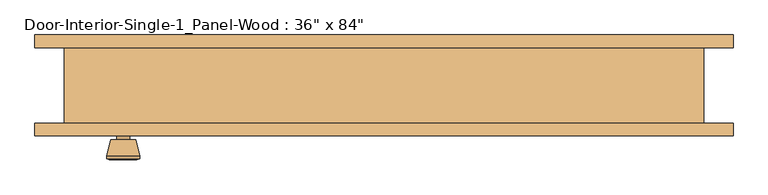
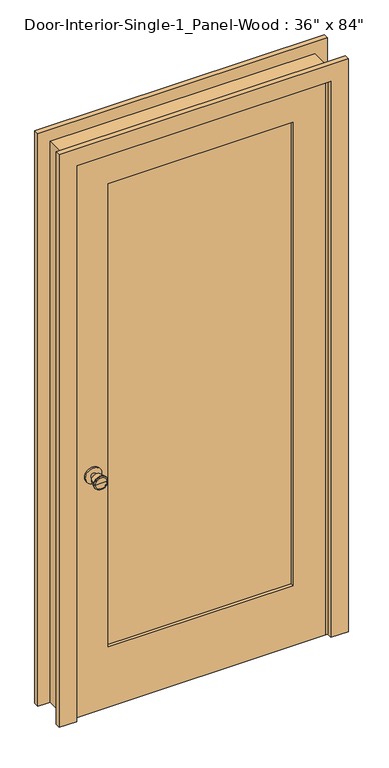
"""IFC4 building model written with IfcOpenShell, lengths in millimetres: door geometry."""

from ifc_helpers import new_model, si_unit, point, frame, frame_2d, origin, place, context, project, spatial, polyline, circle_curve, trimmed, segment, composite_curve, outline, extrude, faceted_brep, source, transform, mapped, element, save
from ifc_brep_helpers import plane_surface, cylinder_surface, revolved_surface, advanced_brep


def door_a3feeac7(model_context):
    return source(origin(), model_context, "Body", "SolidModel", [
        advanced_brep(
        [(-393.7, -13.05, 914.4), (-403.7, -13.05, 914.4), (-383.7, -13.05, 914.4), (-373.2241324, 35.95, 914.4), (-414.1758676, 35.95, 914.4), (-393.7, 35.95, 914.4), (-368.7, 34.1221319, 914.4), (-418.7, 34.1221319, 914.4), (-368.7, 30.6584537, 914.4), (-418.7, 30.6584537, 914.4), (-375.063764, 5.95, 914.4), (-412.336236, 5.95, 914.4), (-383.7, 5.95, 914.4), (-403.7, 5.95, 914.4)],
        [
            (0, 1),
            (1, 2, circle_curve(frame((-393.7, -13.05, 914.4), z_axis=(0.0, -1.0, 0.0), x_axis=(-1.0, 0.0, 0.0)), 10.0)),
            (2, 0),
            (2, 1, circle_curve(frame((-393.7, -13.05, 914.4), z_axis=(0.0, -1.0, 0.0), x_axis=(-1.0, 0.0, 0.0)), 10.0)),
            (3, 4, circle_curve(frame((-393.7, 35.95, 914.4), z_axis=(0.0, 1.0, 0.0), x_axis=(-1.0, 0.0, 0.0)), 20.4758676)),
            (4, 5),
            (5, 3),
            (4, 3, circle_curve(frame((-393.7, 35.95, 914.4), z_axis=(0.0, 1.0, 0.0), x_axis=(-1.0, 0.0, 0.0)), 20.4758676)),
            (6, 7, circle_curve(frame((-393.7, 34.1221319, 914.4), z_axis=(0.0, 1.0, 0.0), x_axis=(-1.0, 0.0, 0.0)), 25.0)),
            (7, 4),
            (3, 6),
            (7, 6, circle_curve(frame((-393.7, 34.1221319, 914.4), z_axis=(0.0, 1.0, 0.0), x_axis=(-1.0, 0.0, 0.0)), 25.0)),
            (8, 9, circle_curve(frame((-393.7, 30.6584537, 914.4), z_axis=(0.0, 1.0, 0.0), x_axis=(-1.0, 0.0, 0.0)), 25.0)),
            (9, 7),
            (6, 8),
            (9, 8, circle_curve(frame((-393.7, 30.6584537, 914.4), z_axis=(0.0, 1.0, 0.0), x_axis=(-1.0, 0.0, 0.0)), 25.0)),
            (10, 11, circle_curve(frame((-393.7, 5.95, 914.4), z_axis=(0.0, 1.0, 0.0), x_axis=(-1.0, 0.0, 0.0)), 18.636236)),
            (11, 9),
            (8, 10),
            (11, 10, circle_curve(frame((-393.7, 5.95, 914.4), z_axis=(0.0, 1.0, 0.0), x_axis=(-1.0, 0.0, 0.0)), 18.636236)),
            (12, 13, circle_curve(frame((-393.7, 5.95, 914.4), z_axis=(0.0, 1.0, 0.0), x_axis=(-1.0, 0.0, 0.0)), 10.0)),
            (13, 11),
            (10, 12),
            (13, 12, circle_curve(frame((-393.7, 5.95, 914.4), z_axis=(0.0, 1.0, 0.0), x_axis=(-1.0, 0.0, 0.0)), 10.0)),
            (1, 13),
            (12, 2),
        ],
        [
            plane_surface(frame((-393.7, -13.05, 914.4), z_axis=(0.0, -1.0, 0.0), x_axis=(-1.0, 0.0, 0.0))),
            plane_surface(frame((-393.7, 35.95, 914.4), z_axis=(0.0, 1.0, 0.0), x_axis=(-1.0, 0.0, 0.0))),
            revolved_surface(polyline([(-414.1758676, 35.95, 914.4), (-418.7, 34.1221319, 914.4)]), (-393.7, -13.05, 914.4), (0.0, -1.0, 0.0)),
            cylinder_surface(frame((-393.7, -13.05, 914.4), z_axis=(0.0, -1.0, 0.0), x_axis=(-1.0, 0.0, 0.0)), 25.0),
            revolved_surface(polyline([(-418.7, 30.6584537, 914.4), (-412.336236, 5.95, 914.4)]), (-393.7, -13.05, 914.4), (0.0, -1.0, 0.0)),
            plane_surface(frame((-393.7, 5.95, 914.4), z_axis=(0.0, -1.0, 0.0), x_axis=(-1.0, 0.0, 0.0))),
            cylinder_surface(frame((-393.7, -13.05, 914.4), z_axis=(0.0, -1.0, 0.0), x_axis=(-1.0, 0.0, 0.0)), 10.0),
        ],
        [
            (0, [[1, 2, 3]]),
            (0, [[-3, 4, -1]]),
            (1, [[5, 6, 7]]),
            (1, [[8, -7, -6]]),
            (2, [[9, 10, -5, 11]]),
            (2, [[12, -11, -8, -10]]),
            (3, [[13, 14, -9, 15]]),
            (3, [[16, -15, -12, -14]]),
            (4, [[17, 18, -13, 19]]),
            (4, [[20, -19, -16, -18]]),
            (5, [[21, 22, -17, 23]]),
            (5, [[24, -23, -20, -22]]),
            (6, [[-2, 25, -21, 26]]),
            (6, [[-4, -26, -24, -25]]),
        ],
    ),
        extrude(outline(composite_curve([segment(trimmed(circle_curve(frame_2d((914.4, -393.7)), 30.0), [point((914.4, -423.7))], [point((914.4, -363.7))], False, "CARTESIAN"), True, "CONTINUOUS"), segment(trimmed(circle_curve(frame_2d((914.4, -393.7)), 30.0), [point((914.4, -363.7))], [point((914.4, -423.7))], False, "CARTESIAN"), True, "CONTINUOUS")], self_intersect=False)), frame((0.0, -19.05, 0.0), z_axis=(0.0, 1.0, 0.0), x_axis=(0.0, 0.0, 1.0)), (0.0, 0.0, 1.0), 6.0),
        advanced_brep(
        [(-393.7, -59.975, 914.4), (-383.7, -59.975, 914.4), (-403.7, -59.975, 914.4), (-373.2241324, -108.975, 914.4), (-393.7, -108.975, 914.4), (-414.1758676, -108.975, 914.4), (-368.7, -107.1471319, 914.4), (-418.7, -107.1471319, 914.4), (-368.7, -103.6834537, 914.4), (-418.7, -103.6834537, 914.4), (-375.063764, -78.975, 914.4), (-412.336236, -78.975, 914.4), (-383.7, -78.975, 914.4), (-403.7, -78.975, 914.4)],
        [
            (0, 1),
            (1, 2, circle_curve(frame((-393.7, -59.975, 914.4), z_axis=(0.0, 1.0, 0.0), x_axis=(-1.0, 0.0, 0.0)), 10.0)),
            (2, 0),
            (2, 1, circle_curve(frame((-393.7, -59.975, 914.4), z_axis=(0.0, 1.0, 0.0), x_axis=(-1.0, 0.0, 0.0)), 10.0)),
            (3, 4),
            (4, 5),
            (5, 3, circle_curve(frame((-393.7, -108.975, 914.4), z_axis=(0.0, -1.0, 0.0), x_axis=(-1.0, 0.0, 0.0)), 20.4758676)),
            (3, 5, circle_curve(frame((-393.7, -108.975, 914.4), z_axis=(0.0, -1.0, 0.0), x_axis=(-1.0, 0.0, 0.0)), 20.4758676)),
            (6, 3),
            (5, 7),
            (7, 6, circle_curve(frame((-393.7, -107.1471319, 914.4), z_axis=(0.0, -1.0, 0.0), x_axis=(-1.0, 0.0, 0.0)), 25.0)),
            (6, 7, circle_curve(frame((-393.7, -107.1471319, 914.4), z_axis=(0.0, -1.0, 0.0), x_axis=(-1.0, 0.0, 0.0)), 25.0)),
            (8, 6),
            (7, 9),
            (9, 8, circle_curve(frame((-393.7, -103.6834537, 914.4), z_axis=(0.0, -1.0, 0.0), x_axis=(-1.0, 0.0, 0.0)), 25.0)),
            (8, 9, circle_curve(frame((-393.7, -103.6834537, 914.4), z_axis=(0.0, -1.0, 0.0), x_axis=(-1.0, 0.0, 0.0)), 25.0)),
            (10, 8),
            (9, 11),
            (11, 10, circle_curve(frame((-393.7, -78.975, 914.4), z_axis=(0.0, -1.0, 0.0), x_axis=(-1.0, 0.0, 0.0)), 18.636236)),
            (10, 11, circle_curve(frame((-393.7, -78.975, 914.4), z_axis=(0.0, -1.0, 0.0), x_axis=(-1.0, 0.0, 0.0)), 18.636236)),
            (12, 10),
            (11, 13),
            (13, 12, circle_curve(frame((-393.7, -78.975, 914.4), z_axis=(0.0, -1.0, 0.0), x_axis=(-1.0, 0.0, 0.0)), 10.0)),
            (12, 13, circle_curve(frame((-393.7, -78.975, 914.4), z_axis=(0.0, -1.0, 0.0), x_axis=(-1.0, 0.0, 0.0)), 10.0)),
            (1, 12),
            (13, 2),
        ],
        [
            plane_surface(frame((-393.7, -59.975, 914.4), z_axis=(0.0, 1.0, 0.0), x_axis=(-1.0, 0.0, 0.0))),
            plane_surface(frame((-393.7, -108.975, 914.4), z_axis=(0.0, -1.0, 0.0), x_axis=(-1.0, 0.0, 0.0))),
            revolved_surface(polyline([(-414.1758676, -108.975, 914.4), (-418.7, -107.1471319, 914.4)]), (-393.7, -59.975, 914.4), (0.0, 1.0, 0.0)),
            cylinder_surface(frame((-393.7, -59.975, 914.4), z_axis=(0.0, 1.0, 0.0), x_axis=(-1.0, 0.0, 0.0)), 25.0),
            revolved_surface(polyline([(-418.7, -103.6834537, 914.4), (-412.336236, -78.975, 914.4)]), (-393.7, -59.975, 914.4), (0.0, 1.0, 0.0)),
            plane_surface(frame((-393.7, -78.975, 914.4), z_axis=(0.0, 1.0, 0.0), x_axis=(-1.0, 0.0, 0.0))),
            cylinder_surface(frame((-393.7, -59.975, 914.4), z_axis=(0.0, 1.0, 0.0), x_axis=(-1.0, 0.0, 0.0)), 10.0),
        ],
        [
            (0, [[1, 2, 3]]),
            (0, [[-3, 4, -1]]),
            (1, [[5, 6, 7]]),
            (1, [[-6, -5, 8]]),
            (2, [[9, -7, 10, 11]]),
            (2, [[-10, -8, -9, 12]]),
            (3, [[13, -11, 14, 15]]),
            (3, [[-14, -12, -13, 16]]),
            (4, [[17, -15, 18, 19]]),
            (4, [[-18, -16, -17, 20]]),
            (5, [[21, -19, 22, 23]]),
            (5, [[-22, -20, -21, 24]]),
            (6, [[25, -23, 26, -2]]),
            (6, [[-26, -24, -25, -4]]),
        ],
    ),
        extrude(outline(composite_curve([segment(trimmed(circle_curve(frame_2d((914.4, -393.7)), 30.0), [point((914.4, -423.7))], [point((914.4, -363.7))], False, "CARTESIAN"), True, "CONTINUOUS"), segment(trimmed(circle_curve(frame_2d((914.4, -393.7)), 30.0), [point((914.4, -363.7))], [point((914.4, -423.7))], False, "CARTESIAN"), True, "CONTINUOUS")], self_intersect=False)), frame((0.0, -59.975, 0.0), z_axis=(0.0, 1.0, 0.0), x_axis=(0.0, 0.0, 1.0)), (0.0, 0.0, 1.0), 6.0),
        faceted_brep([(482.6, -53.975, 0.0), (457.2, -53.975, 0.0), (457.2, -19.05, 0.0), (444.5, -19.05, 0.0), (444.5, 15.875, 0.0), (457.2, 15.875, 0.0), (457.2, 60.325, 0.0), (482.6, 60.325, 0.0), (482.6, 60.325, 2159.0), (482.6, -53.975, 2159.0), (457.2, 60.325, 2133.6), (-457.2, 60.325, 2133.6), (-457.2, 60.325, 0.0), (-482.6, 60.325, 0.0), (-482.6, 60.325, 2159.0), (457.2, 15.875, 2133.6), (444.5, 15.875, 2120.9), (-444.5, 15.875, 2120.9), (-444.5, 15.875, 0.0), (-457.2, 15.875, 0.0), (-457.2, 15.875, 2133.6), (444.5, -19.05, 2120.9), (457.2, -19.05, 2133.6), (-457.2, -19.05, 2133.6), (-457.2, -19.05, 0.0), (-444.5, -19.05, 0.0), (-444.5, -19.05, 2120.9), (457.2, -53.975, 2133.6), (-482.6, -53.975, 2159.0), (-482.6, -53.975, 0.0), (-457.2, -53.975, 0.0), (-457.2, -53.975, 2133.6)], [[[0, 1, 2, 3, 4, 5, 6, 7]], [[7, 8, 9, 0]], [[6, 10, 11, 12, 13, 14, 8, 7]], [[5, 15, 10, 6]], [[4, 16, 17, 18, 19, 20, 15, 5]], [[3, 21, 16, 4]], [[2, 22, 23, 24, 25, 26, 21, 3]], [[1, 27, 22, 2]], [[0, 9, 28, 29, 30, 31, 27, 1]], [[8, 14, 28, 9]], [[15, 20, 11, 10]], [[21, 26, 17, 16]], [[27, 31, 23, 22]], [[29, 13, 12, 19, 18, 25, 24, 30]], [[14, 13, 29, 28]], [[20, 19, 12, 11]], [[26, 25, 18, 17]], [[31, 30, 24, 23]]]),
        extrude(outline(polyline([(2133.6, -457.2), (0.0, -457.2), (0.0, 457.2), (2133.6, 457.2), (2133.6, -457.2)]), holes=[polyline([(2014.5375, -336.55), (2014.5375, 336.55), (231.775, 336.55), (231.775, -336.55), (2014.5375, -336.55)])]), frame((0.0, -53.975, 0.0), z_axis=(0.0, 1.0, 0.0), x_axis=(0.0, 0.0, 1.0)), (0.0, 0.0, 1.0), 34.925),
        extrude(outline(polyline([(336.55, -30.6916667), (336.55, -42.3333333), (-336.55, -42.3333333), (-336.55, -30.6916667), (336.55, -30.6916667)])), frame((0.0, 0.0, 231.775), z_axis=(0.0, 0.0, 1.0), x_axis=(1.0, 0.0, 0.0)), (0.0, 0.0, 1.0), 1782.7625),
        extrude(outline(polyline([(0.0, 527.05), (2203.45, 527.05), (2203.45, -527.05), (0.0, -527.05), (0.0, -463.55), (2139.95, -463.55), (2139.95, 463.55), (0.0, 463.55), (0.0, 527.05)])), frame((0.0, -73.025, 0.0), z_axis=(0.0, 1.0, 0.0), x_axis=(0.0, 0.0, 1.0)), (0.0, 0.0, 1.0), 19.05),
        extrude(outline(polyline([(0.0, 527.05), (2203.45, 527.05), (2203.45, -527.05), (0.0, -527.05), (0.0, -463.55), (2139.95, -463.55), (2139.95, 463.55), (0.0, 463.55), (0.0, 527.05)])), frame((0.0, 60.325, 0.0), z_axis=(0.0, 1.0, 0.0), x_axis=(0.0, 0.0, 1.0)), (0.0, 0.0, 1.0), 19.05),
    ])


if __name__ == "__main__":
    model = new_model("IFC4")
    model_context = context("Model", 3, world=origin())
    ifc_project = project(units=[si_unit("LENGTHUNIT", "METRE", prefix="MILLI")], contexts=[model_context])
    site = spatial("IfcSite", under=ifc_project)
    building = spatial("IfcBuilding", under=site)
    placement = place(None, origin())
    door_shape = door_a3feeac7(model_context)
    element("IfcDoor", 1, ObjectType="Door-Interior-Single-1_Panel-Wood : 36\" x 84\"", at=placement, inside=building, context=model_context, shape_type="MappedRepresentation", body=[
        mapped(door_shape, transform((0.0, 0.0, 0.0), x_axis=(1.0, 0.0, 0.0), y_axis=(0.0, 1.0, 0.0), z_axis=(0.0, 0.0, 1.0))),
    ])
    save(model, "model.ifc")

# Revit data of these elements
# Type "Door-Interior-Single-1_Panel-Wood : 36\" x 84\""
#   Type Mark = "15"
#   Assembly Code = "C1020300"
#   Analytic Construction = "Wooden"
#   Top Rail = 0' - 4 11/16"
#   Thickness = 0' - 1 3/8"
#   Thermal Resistance (R) = 2.5876 (h·ft²·°F)/BTU
#   Swing Angle [instance default] = 90.00°
#   Stiles = 0' - 4 3/4"
#   Rough Width = 3' - 2"
#   Rough Height = 7' - 1"
#   Height = 7' - 0"
#   Width = 3' - 0"
#   Heat Transfer Coefficient (U) = 0.3865 BTU/(h·ft²·°F)
#   Bottom Rail = 0' - 9 1/8"
#   Trim Material = Cherry
#   Panel Material = Cherry
#   Frame Material = Cherry
#   Door Handle Material = Aluminum
#   Visual Light Transmittance = 0
#   Solar Heat Gain Coefficient = 0
#   Wall Closure = (empty or 0)
#   Function = (empty or 0)
# Element 1 (IfcDoor, "Door-Interior-Single-1_Panel-Wood : 36\" x 84\"")
#   Materials on its faces: "Cherry", "Aluminum"
# Materials
#   "Cherry": class "Wood", colour RGB 226 177 128, transparency 0, Description = "Prunus Serotina", Cost = 0
#   "Aluminum": class "Metal", colour RGB 247 247 247, transparency 0, Description = "Aluminum 6061", Cost = 0
